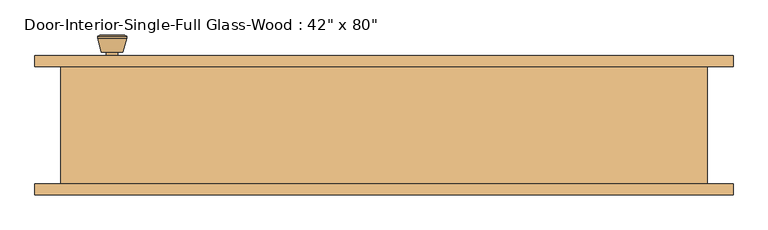
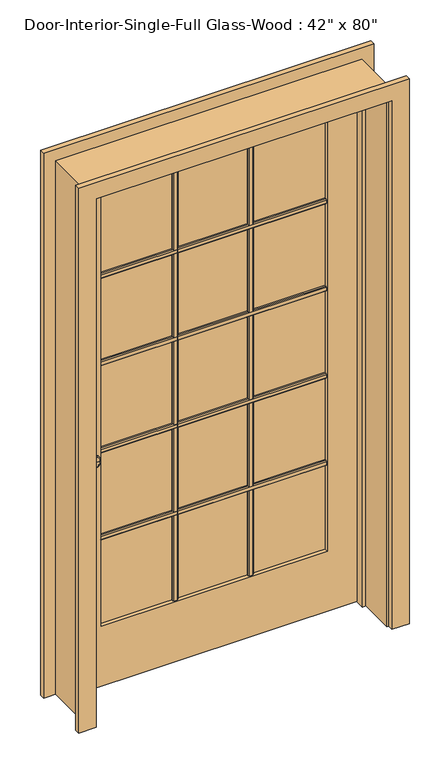
"""IFC4 building model written with IfcOpenShell, lengths in millimetres: door geometry."""

from ifc_helpers import new_model, si_unit, point, frame, frame_2d, origin, place, context, project, spatial, polyline, circle_curve, trimmed, segment, composite_curve, outline, extrude, faceted_brep, source, transform, mapped, element, save
from ifc_brep_helpers import plane_surface, cylinder_surface, revolved_surface, advanced_brep


def door_f3911013(model_context):
    return source(origin(), model_context, "Body", "SolidModel", [
        extrude(outline(polyline([(84.455, 1586.23), (90.805, 1586.23), (93.98, 1583.055), (93.98, 1570.355), (90.805, 1567.18), (84.455, 1567.18), (84.455, 1586.23)])), frame((-412.75, 0.0, 0.0), z_axis=(1.0, 0.0, 0.0), x_axis=(0.0, 1.0, 0.0)), (0.0, 0.0, 1.0), 825.5),
        extrude(outline(polyline([(84.455, 1249.9975), (90.805, 1249.9975), (93.98, 1246.8225), (93.98, 1234.1225), (90.805, 1230.9475), (84.455, 1230.9475), (84.455, 1249.9975)])), frame((-412.75, 0.0, 0.0), z_axis=(1.0, 0.0, 0.0), x_axis=(0.0, 1.0, 0.0)), (0.0, 0.0, 1.0), 825.5),
        extrude(outline(polyline([(84.455, 913.765), (90.805, 913.765), (93.98, 910.59), (93.98, 897.89), (90.805, 894.715), (84.455, 894.715), (84.455, 913.765)])), frame((-412.75, 0.0, 0.0), z_axis=(1.0, 0.0, 0.0), x_axis=(0.0, 1.0, 0.0)), (0.0, 0.0, 1.0), 825.5),
        extrude(outline(polyline([(84.455, 577.5325), (90.805, 577.5325), (93.98, 574.3575), (93.98, 561.6575), (90.805, 558.4825), (84.455, 558.4825), (84.455, 577.5325)])), frame((-412.75, 0.0, 0.0), z_axis=(1.0, 0.0, 0.0), x_axis=(0.0, 1.0, 0.0)), (0.0, 0.0, 1.0), 825.5),
        extrude(outline(polyline([(128.0583333, 84.455), (128.0583333, 90.805), (131.2333333, 93.98), (143.9333333, 93.98), (147.1083333, 90.805), (147.1083333, 84.455), (128.0583333, 84.455)])), frame((0.0, 0.0, 231.775), z_axis=(0.0, 0.0, 1.0), x_axis=(1.0, 0.0, 0.0)), (0.0, 0.0, 1.0), 1681.1625),
        extrude(outline(polyline([(-147.1083333, 84.455), (-147.1083333, 90.805), (-143.9333333, 93.98), (-131.2333333, 93.98), (-128.0583333, 90.805), (-128.0583333, 84.455), (-147.1083333, 84.455)])), frame((0.0, 0.0, 231.775), z_axis=(0.0, 0.0, 1.0), x_axis=(1.0, 0.0, 0.0)), (0.0, 0.0, 1.0), 1681.1625),
        extrude(outline(polyline([(77.47, 1586.23), (77.47, 1567.18), (71.12, 1567.18), (67.945, 1570.355), (67.945, 1583.055), (71.12, 1586.23), (77.47, 1586.23)])), frame((-412.75, 0.0, 0.0), z_axis=(1.0, 0.0, 0.0), x_axis=(0.0, 1.0, 0.0)), (0.0, 0.0, 1.0), 825.5),
        extrude(outline(polyline([(77.47, 1249.9975), (77.47, 1230.9475), (71.12, 1230.9475), (67.945, 1234.1225), (67.945, 1246.8225), (71.12, 1249.9975), (77.47, 1249.9975)])), frame((-412.75, 0.0, 0.0), z_axis=(1.0, 0.0, 0.0), x_axis=(0.0, 1.0, 0.0)), (0.0, 0.0, 1.0), 825.5),
        extrude(outline(polyline([(77.47, 913.765), (77.47, 894.715), (71.12, 894.715), (67.945, 897.89), (67.945, 910.59), (71.12, 913.765), (77.47, 913.765)])), frame((-412.75, 0.0, 0.0), z_axis=(1.0, 0.0, 0.0), x_axis=(0.0, 1.0, 0.0)), (0.0, 0.0, 1.0), 825.5),
        extrude(outline(polyline([(77.47, 577.5325), (77.47, 558.4825), (71.12, 558.4825), (67.945, 561.6575), (67.945, 574.3575), (71.12, 577.5325), (77.47, 577.5325)])), frame((-412.75, 0.0, 0.0), z_axis=(1.0, 0.0, 0.0), x_axis=(0.0, 1.0, 0.0)), (0.0, 0.0, 1.0), 825.5),
        extrude(outline(polyline([(128.0583333, 77.47), (147.1083333, 77.47), (147.1083333, 71.12), (143.9333333, 67.945), (131.2333333, 67.945), (128.0583333, 71.12), (128.0583333, 77.47)])), frame((0.0, 0.0, 231.775), z_axis=(0.0, 0.0, 1.0), x_axis=(1.0, 0.0, 0.0)), (0.0, 0.0, 1.0), 1681.1625),
        extrude(outline(polyline([(-147.1083333, 77.47), (-128.0583333, 77.47), (-128.0583333, 71.12), (-131.2333333, 67.945), (-143.9333333, 67.945), (-147.1083333, 71.12), (-147.1083333, 77.47)])), frame((0.0, 0.0, 231.775), z_axis=(0.0, 0.0, 1.0), x_axis=(1.0, 0.0, 0.0)), (0.0, 0.0, 1.0), 1681.1625),
        advanced_brep(
        [(-469.9, 57.5, 914.4), (-459.9, 57.5, 914.4), (-479.9, 57.5, 914.4), (-449.4241324, 8.5, 914.4), (-469.9, 8.5, 914.4), (-490.3758676, 8.5, 914.4), (-444.9, 10.3278681, 914.4), (-494.9, 10.3278681, 914.4), (-444.9, 13.7915463, 914.4), (-494.9, 13.7915463, 914.4), (-451.263764, 38.5, 914.4), (-488.536236, 38.5, 914.4), (-459.9, 38.5, 914.4), (-479.9, 38.5, 914.4)],
        [
            (0, 1),
            (1, 2, circle_curve(frame((-469.9, 57.5, 914.4), z_axis=(0.0, 1.0, 0.0), x_axis=(-1.0, 0.0, 0.0)), 10.0)),
            (2, 0),
            (2, 1, circle_curve(frame((-469.9, 57.5, 914.4), z_axis=(0.0, 1.0, 0.0), x_axis=(-1.0, 0.0, 0.0)), 10.0)),
            (3, 4),
            (4, 5),
            (5, 3, circle_curve(frame((-469.9, 8.5, 914.4), z_axis=(0.0, -1.0, 0.0), x_axis=(-1.0, 0.0, 0.0)), 20.4758676)),
            (3, 5, circle_curve(frame((-469.9, 8.5, 914.4), z_axis=(0.0, -1.0, 0.0), x_axis=(-1.0, 0.0, 0.0)), 20.4758676)),
            (6, 3),
            (5, 7),
            (7, 6, circle_curve(frame((-469.9, 10.3278681, 914.4), z_axis=(0.0, -1.0, 0.0), x_axis=(-1.0, 0.0, 0.0)), 25.0)),
            (6, 7, circle_curve(frame((-469.9, 10.3278681, 914.4), z_axis=(0.0, -1.0, 0.0), x_axis=(-1.0, 0.0, 0.0)), 25.0)),
            (8, 6),
            (7, 9),
            (9, 8, circle_curve(frame((-469.9, 13.7915463, 914.4), z_axis=(0.0, -1.0, 0.0), x_axis=(-1.0, 0.0, 0.0)), 25.0)),
            (8, 9, circle_curve(frame((-469.9, 13.7915463, 914.4), z_axis=(0.0, -1.0, 0.0), x_axis=(-1.0, 0.0, 0.0)), 25.0)),
            (10, 8),
            (9, 11),
            (11, 10, circle_curve(frame((-469.9, 38.5, 914.4), z_axis=(0.0, -1.0, 0.0), x_axis=(-1.0, 0.0, 0.0)), 18.636236)),
            (10, 11, circle_curve(frame((-469.9, 38.5, 914.4), z_axis=(0.0, -1.0, 0.0), x_axis=(-1.0, 0.0, 0.0)), 18.636236)),
            (12, 10),
            (11, 13),
            (13, 12, circle_curve(frame((-469.9, 38.5, 914.4), z_axis=(0.0, -1.0, 0.0), x_axis=(-1.0, 0.0, 0.0)), 10.0)),
            (12, 13, circle_curve(frame((-469.9, 38.5, 914.4), z_axis=(0.0, -1.0, 0.0), x_axis=(-1.0, 0.0, 0.0)), 10.0)),
            (1, 12),
            (13, 2),
        ],
        [
            plane_surface(frame((-469.9, 57.5, 914.4), z_axis=(0.0, 1.0, 0.0), x_axis=(-1.0, 0.0, 0.0))),
            plane_surface(frame((-469.9, 8.5, 914.4), z_axis=(0.0, -1.0, 0.0), x_axis=(-1.0, 0.0, 0.0))),
            revolved_surface(polyline([(-490.3758676, 8.5, 914.4), (-494.9, 10.3278681, 914.4)]), (-469.9, 57.5, 914.4), (0.0, 1.0, 0.0)),
            cylinder_surface(frame((-469.9, 57.5, 914.4), z_axis=(0.0, 1.0, 0.0), x_axis=(-1.0, 0.0, 0.0)), 25.0),
            revolved_surface(polyline([(-494.9, 13.7915463, 914.4), (-488.536236, 38.5, 914.4)]), (-469.9, 57.5, 914.4), (0.0, 1.0, 0.0)),
            plane_surface(frame((-469.9, 38.5, 914.4), z_axis=(0.0, 1.0, 0.0), x_axis=(-1.0, 0.0, 0.0))),
            cylinder_surface(frame((-469.9, 57.5, 914.4), z_axis=(0.0, 1.0, 0.0), x_axis=(-1.0, 0.0, 0.0)), 10.0),
        ],
        [
            (0, [[1, 2, 3]]),
            (0, [[-3, 4, -1]]),
            (1, [[5, 6, 7]]),
            (1, [[-6, -5, 8]]),
            (2, [[9, -7, 10, 11]]),
            (2, [[-10, -8, -9, 12]]),
            (3, [[13, -11, 14, 15]]),
            (3, [[-14, -12, -13, 16]]),
            (4, [[17, -15, 18, 19]]),
            (4, [[-18, -16, -17, 20]]),
            (5, [[21, -19, 22, 23]]),
            (5, [[-22, -20, -21, 24]]),
            (6, [[25, -23, 26, -2]]),
            (6, [[-26, -24, -25, -4]]),
        ],
    ),
        extrude(outline(composite_curve([segment(trimmed(circle_curve(frame_2d((914.4, -469.9)), 30.0), [point((914.4, -499.9))], [point((914.4, -439.9))], False, "CARTESIAN"), True, "CONTINUOUS"), segment(trimmed(circle_curve(frame_2d((914.4, -469.9)), 30.0), [point((914.4, -439.9))], [point((914.4, -499.9))], False, "CARTESIAN"), True, "CONTINUOUS")], self_intersect=False)), frame((0.0, 57.5, 0.0), z_axis=(0.0, 1.0, 0.0), x_axis=(0.0, 0.0, 1.0)), (0.0, 0.0, 1.0), 6.0),
        advanced_brep(
        [(-469.9, 104.425, 914.4), (-479.9, 104.425, 914.4), (-459.9, 104.425, 914.4), (-449.4241324, 153.425, 914.4), (-490.3758676, 153.425, 914.4), (-469.9, 153.425, 914.4), (-444.9, 151.5971319, 914.4), (-494.9, 151.5971319, 914.4), (-444.9, 148.1334537, 914.4), (-494.9, 148.1334537, 914.4), (-451.263764, 123.425, 914.4), (-488.536236, 123.425, 914.4), (-459.9, 123.425, 914.4), (-479.9, 123.425, 914.4)],
        [
            (0, 1),
            (1, 2, circle_curve(frame((-469.9, 104.425, 914.4), z_axis=(0.0, -1.0, 0.0), x_axis=(-1.0, 0.0, 0.0)), 10.0)),
            (2, 0),
            (2, 1, circle_curve(frame((-469.9, 104.425, 914.4), z_axis=(0.0, -1.0, 0.0), x_axis=(-1.0, 0.0, 0.0)), 10.0)),
            (3, 4, circle_curve(frame((-469.9, 153.425, 914.4), z_axis=(0.0, 1.0, 0.0), x_axis=(-1.0, 0.0, 0.0)), 20.4758676)),
            (4, 5),
            (5, 3),
            (4, 3, circle_curve(frame((-469.9, 153.425, 914.4), z_axis=(0.0, 1.0, 0.0), x_axis=(-1.0, 0.0, 0.0)), 20.4758676)),
            (6, 7, circle_curve(frame((-469.9, 151.5971319, 914.4), z_axis=(0.0, 1.0, 0.0), x_axis=(-1.0, 0.0, 0.0)), 25.0)),
            (7, 4),
            (3, 6),
            (7, 6, circle_curve(frame((-469.9, 151.5971319, 914.4), z_axis=(0.0, 1.0, 0.0), x_axis=(-1.0, 0.0, 0.0)), 25.0)),
            (8, 9, circle_curve(frame((-469.9, 148.1334537, 914.4), z_axis=(0.0, 1.0, 0.0), x_axis=(-1.0, 0.0, 0.0)), 25.0)),
            (9, 7),
            (6, 8),
            (9, 8, circle_curve(frame((-469.9, 148.1334537, 914.4), z_axis=(0.0, 1.0, 0.0), x_axis=(-1.0, 0.0, 0.0)), 25.0)),
            (10, 11, circle_curve(frame((-469.9, 123.425, 914.4), z_axis=(0.0, 1.0, 0.0), x_axis=(-1.0, 0.0, 0.0)), 18.636236)),
            (11, 9),
            (8, 10),
            (11, 10, circle_curve(frame((-469.9, 123.425, 914.4), z_axis=(0.0, 1.0, 0.0), x_axis=(-1.0, 0.0, 0.0)), 18.636236)),
            (12, 13, circle_curve(frame((-469.9, 123.425, 914.4), z_axis=(0.0, 1.0, 0.0), x_axis=(-1.0, 0.0, 0.0)), 10.0)),
            (13, 11),
            (10, 12),
            (13, 12, circle_curve(frame((-469.9, 123.425, 914.4), z_axis=(0.0, 1.0, 0.0), x_axis=(-1.0, 0.0, 0.0)), 10.0)),
            (1, 13),
            (12, 2),
        ],
        [
            plane_surface(frame((-469.9, 104.425, 914.4), z_axis=(0.0, -1.0, 0.0), x_axis=(-1.0, 0.0, 0.0))),
            plane_surface(frame((-469.9, 153.425, 914.4), z_axis=(0.0, 1.0, 0.0), x_axis=(-1.0, 0.0, 0.0))),
            revolved_surface(polyline([(-490.3758676, 153.425, 914.4), (-494.9, 151.5971319, 914.4)]), (-469.9, 104.425, 914.4), (0.0, -1.0, 0.0)),
            cylinder_surface(frame((-469.9, 104.425, 914.4), z_axis=(0.0, -1.0, 0.0), x_axis=(-1.0, 0.0, 0.0)), 25.0),
            revolved_surface(polyline([(-494.9, 148.1334537, 914.4), (-488.536236, 123.425, 914.4)]), (-469.9, 104.425, 914.4), (0.0, -1.0, 0.0)),
            plane_surface(frame((-469.9, 123.425, 914.4), z_axis=(0.0, -1.0, 0.0), x_axis=(-1.0, 0.0, 0.0))),
            cylinder_surface(frame((-469.9, 104.425, 914.4), z_axis=(0.0, -1.0, 0.0), x_axis=(-1.0, 0.0, 0.0)), 10.0),
        ],
        [
            (0, [[1, 2, 3]]),
            (0, [[-3, 4, -1]]),
            (1, [[5, 6, 7]]),
            (1, [[8, -7, -6]]),
            (2, [[9, 10, -5, 11]]),
            (2, [[12, -11, -8, -10]]),
            (3, [[13, 14, -9, 15]]),
            (3, [[16, -15, -12, -14]]),
            (4, [[17, 18, -13, 19]]),
            (4, [[20, -19, -16, -18]]),
            (5, [[21, 22, -17, 23]]),
            (5, [[24, -23, -20, -22]]),
            (6, [[-2, 25, -21, 26]]),
            (6, [[-4, -26, -24, -25]]),
        ],
    ),
        extrude(outline(composite_curve([segment(trimmed(circle_curve(frame_2d((914.4, -469.9)), 30.0), [point((914.4, -499.9))], [point((914.4, -439.9))], False, "CARTESIAN"), True, "CONTINUOUS"), segment(trimmed(circle_curve(frame_2d((914.4, -469.9)), 30.0), [point((914.4, -439.9))], [point((914.4, -499.9))], False, "CARTESIAN"), True, "CONTINUOUS")], self_intersect=False)), frame((0.0, 98.425, 0.0), z_axis=(0.0, 1.0, 0.0), x_axis=(0.0, 0.0, 1.0)), (0.0, 0.0, 1.0), 6.0),
        extrude(outline(polyline([(2032.0, -533.4), (0.0, -533.4), (0.0, 533.4), (2032.0, 533.4), (2032.0, -533.4)]), holes=[polyline([(1912.9375, -412.75), (1912.9375, 412.75), (231.775, 412.75), (231.775, -412.75), (1912.9375, -412.75)])]), frame((0.0, 63.5, 0.0), z_axis=(0.0, 1.0, 0.0), x_axis=(0.0, 0.0, 1.0)), (0.0, 0.0, 1.0), 34.925),
        faceted_brep([(558.8, 98.425, 0.0), (558.8, -104.775, 0.0), (533.4, -104.775, 0.0), (533.4, 28.575, 0.0), (520.7, 28.575, 0.0), (520.7, 63.5, 0.0), (533.4, 63.5, 0.0), (533.4, 98.425, 0.0), (558.8, 98.425, 2057.4), (558.8, -104.775, 2057.4), (-558.8, -104.775, 2057.4), (-558.8, -104.775, 0.0), (-533.4, -104.775, 0.0), (-533.4, -104.775, 2032.0), (533.4, -104.775, 2032.0), (533.4, 28.575, 2032.0), (-533.4, 28.575, 2032.0), (-533.4, 28.575, 0.0), (-520.7, 28.575, 0.0), (-520.7, 28.575, 2019.3), (520.7, 28.575, 2019.3), (520.7, 63.5, 2019.3), (-520.7, 63.5, 2019.3), (-520.7, 63.5, 0.0), (-533.4, 63.5, 0.0), (-533.4, 63.5, 2032.0), (533.4, 63.5, 2032.0), (533.4, 98.425, 2032.0), (-533.4, 98.425, 2032.0), (-533.4, 98.425, 0.0), (-558.8, 98.425, 0.0), (-558.8, 98.425, 2057.4)], [[[0, 1, 2, 3, 4, 5, 6, 7]], [[1, 0, 8, 9]], [[2, 1, 9, 10, 11, 12, 13, 14]], [[3, 2, 14, 15]], [[4, 3, 15, 16, 17, 18, 19, 20]], [[5, 4, 20, 21]], [[6, 5, 21, 22, 23, 24, 25, 26]], [[7, 6, 26, 27]], [[0, 7, 27, 28, 29, 30, 31, 8]], [[9, 8, 31, 10]], [[15, 14, 13, 16]], [[21, 20, 19, 22]], [[27, 26, 25, 28]], [[30, 29, 24, 23, 18, 17, 12, 11]], [[10, 31, 30, 11]], [[16, 13, 12, 17]], [[22, 19, 18, 23]], [[28, 25, 24, 29]]]),
        extrude(outline(polyline([(412.75, 77.47), (-412.75, 77.47), (-412.75, 84.455), (412.75, 84.455), (412.75, 77.47)])), frame((0.0, 0.0, 231.775), z_axis=(0.0, 0.0, 1.0), x_axis=(1.0, 0.0, 0.0)), (0.0, 0.0, 1.0), 1681.1625),
        extrude(outline(polyline([(0.0, 539.75), (0.0, 603.25), (2101.85, 603.25), (2101.85, -603.25), (0.0, -603.25), (0.0, -539.75), (2038.35, -539.75), (2038.35, 539.75), (0.0, 539.75)])), frame((0.0, -123.825, 0.0), z_axis=(0.0, 1.0, 0.0), x_axis=(0.0, 0.0, 1.0)), (0.0, 0.0, 1.0), 19.05),
        extrude(outline(polyline([(0.0, 539.75), (0.0, 603.25), (2101.85, 603.25), (2101.85, -603.25), (0.0, -603.25), (0.0, -539.75), (2038.35, -539.75), (2038.35, 539.75), (0.0, 539.75)])), frame((0.0, 98.425, 0.0), z_axis=(0.0, 1.0, 0.0), x_axis=(0.0, 0.0, 1.0)), (0.0, 0.0, 1.0), 19.05),
    ])


if __name__ == "__main__":
    model = new_model("IFC4")
    model_context = context("Model", 3, world=origin())
    ifc_project = project(units=[si_unit("LENGTHUNIT", "METRE", prefix="MILLI")], contexts=[model_context])
    site = spatial("IfcSite", under=ifc_project)
    building = spatial("IfcBuilding", under=site)
    placement = place(None, origin())
    door_shape = door_f3911013(model_context)
    element("IfcDoor", 1, ObjectType="Door-Interior-Single-Full Glass-Wood : 42\" x 80\"", at=placement, inside=building, context=model_context, shape_type="MappedRepresentation", body=[
        mapped(door_shape, transform((0.0, 0.0, 0.0), x_axis=(1.0, 0.0, 0.0), y_axis=(0.0, 1.0, 0.0), z_axis=(0.0, 0.0, 1.0))),
    ])
    save(model, "model.ifc")

# Revit data of these elements
# Type "Door-Interior-Single-Full Glass-Wood : 42\" x 80\""
#   Type Mark = "19"
#   Assembly Code = "C1020300"
#   Analytic Construction = "Wood frame with single clear glass"
#   Top Rail = 0' - 4 11/16"
#   Thickness = 0' - 1 3/8"
#   Thermal Resistance (R) = 1.0102 (h·ft²·°F)/BTU
#   Swing Angle [instance default] = 90.00°
#   Stiles = 0' - 4 3/4"
#   Rough Width = 3' - 8"
#   Rough Height = 6' - 9"
#   Height = 6' - 8"
#   Width = 3' - 6"
#   Heat Transfer Coefficient (U) = 0.9900 BTU/(h·ft²·°F)
#   Bottom Rail = 0' - 9 1/8"
#   Show Grill [instance default] = yes
#   Trim Material = Cherry
#   Panel Material = Cherry
#   Frame Material = Cherry
#   Door Handle Material = Aluminum
#   Visual Light Transmittance = 0
#   Solar Heat Gain Coefficient = 0
#   Wall Closure = (empty or 0)
#   Function = (empty or 0)
# Element 1 (IfcDoor, "Door-Interior-Single-Full Glass-Wood : 42\" x 80\"")
#   Materials on its faces: "Cherry", "Aluminum", "Glass"
# Materials
#   "Cherry": class "Wood", colour RGB 226 177 128, transparency 0, Description = "Prunus Serotina", Cost = 0
#   "Aluminum": class "Metal", colour RGB 247 247 247, transparency 0, Description = "Aluminum 6061", Cost = 0
#   "Glass": class "Glass", colour RGB 0 128 192, transparency 0.75, Description = "Soda Lime Glass", Cost = 0
